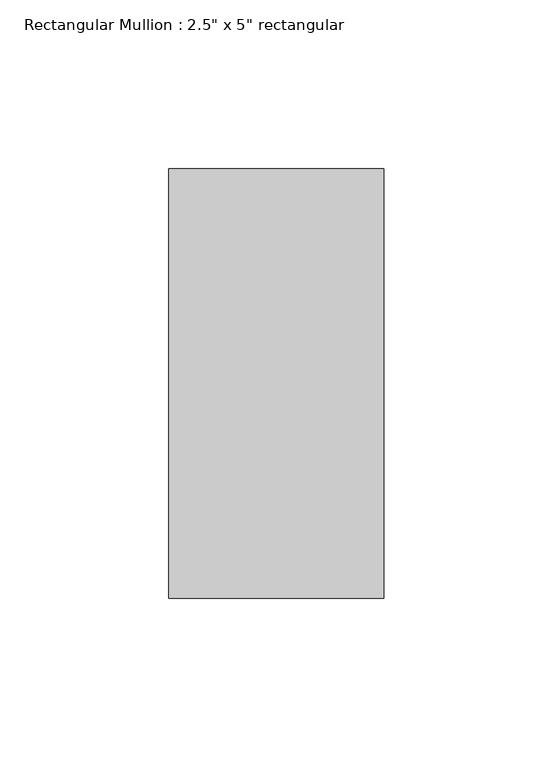
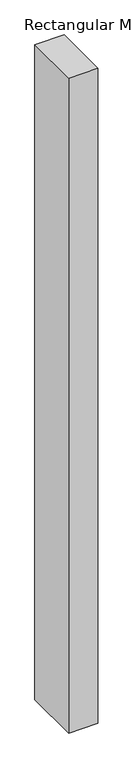
"""IFC4 building model written with IfcOpenShell, lengths in millimetres: member geometry."""

from ifc_helpers import new_model, si_unit, frame, origin, place, context, project, spatial, polyline, outline, extrude, source, transform, mapped, element, save


def member_3586d5c2(model_context):
    return source(origin(), model_context, "Body", "SweptSolid", [
        extrude(outline(polyline([(31.75, 63.5), (31.75, -63.5), (-31.75, -63.5), (-31.75, 63.5), (31.75, 63.5)])), frame((0.0, 0.0, -1506.17602), z_axis=(0.0, 0.0, 1.0), x_axis=(1.0, 0.0, 0.0)), (0.0, 0.0, 1.0), 1506.17602),
    ])


if __name__ == "__main__":
    model = new_model("IFC4")
    model_context = context("Model", 3, world=origin())
    ifc_project = project(units=[si_unit("LENGTHUNIT", "METRE", prefix="MILLI")], contexts=[model_context])
    site = spatial("IfcSite", under=ifc_project)
    building = spatial("IfcBuilding", under=site)
    placement = place(None, origin())
    member_shape = member_3586d5c2(model_context)
    element("IfcMember", 1, ObjectType="Rectangular Mullion : 2.5\" x 5\" rectangular", at=placement, inside=building, context=model_context, shape_type="MappedRepresentation", body=[
        mapped(member_shape, transform((0.0, 0.0, 0.0), x_axis=(1.0, 0.0, 0.0), y_axis=(0.0, 1.0, 0.0), z_axis=(0.0, 0.0, 1.0))),
    ])
    save(model, "model.ifc")

# Revit data of these elements
# Type "Rectangular Mullion : 2.5\" x 5\" rectangular"
#   built-in parameter 1007304 = 0.416667 (stored number, unit not read)
#   built-in parameter 1007301 = 0.104167 (stored number, unit not read)
#   built-in parameter 1007300 = 0.104167 (stored number, unit not read)
# Element 1 (IfcMember, "Rectangular Mullion : 2.5\" x 5\" rectangular")
#   Materials on its faces: "Aluminum"
# Materials
#   "Aluminum": class "Metal", colour RGB 247 247 247, transparency 0, Description = "Aluminum 6061", Cost = 0
